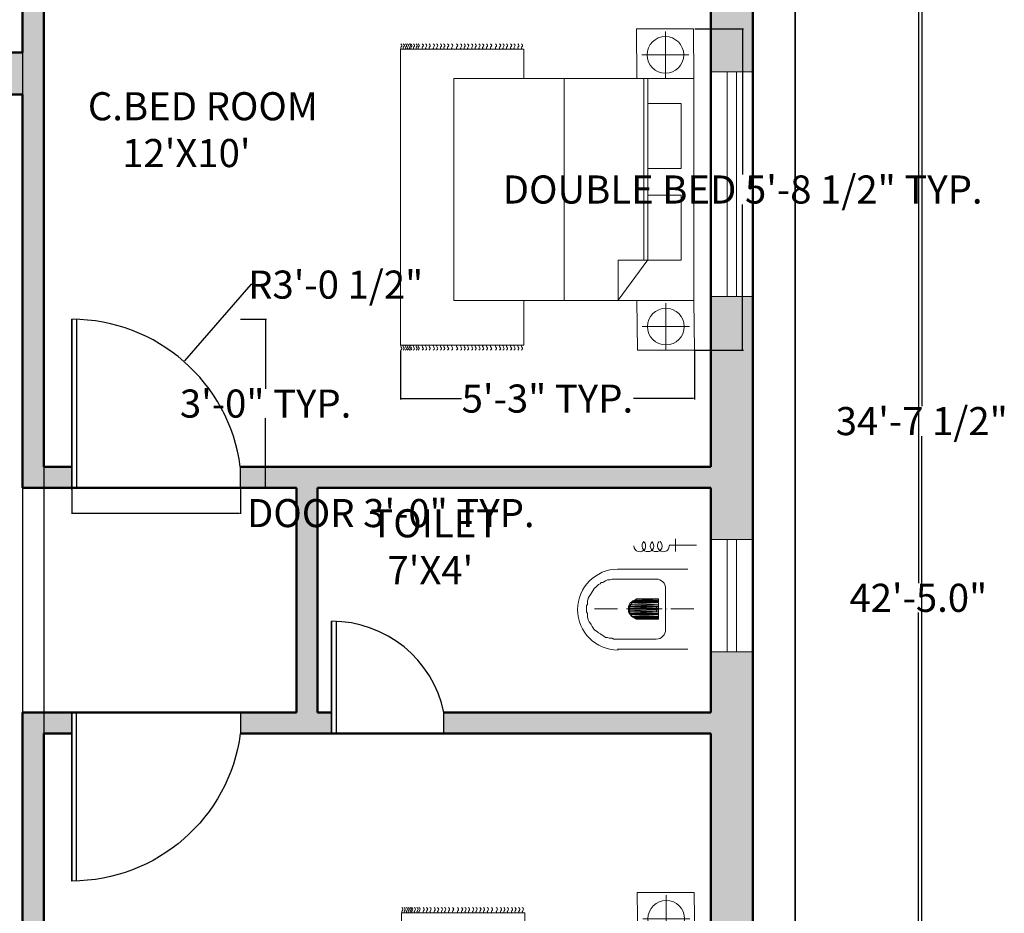
# Model space of a CAD drawing. Units: inches. Extents: x 3398 to 3816, y 15195 to 15771.
# Tile 8 of 10: x 3606 to 3816, y 15418 to 15609. Entities that reach past the tile are written whole.
import ezdxf

# ---------------------------------------------------------------- set-up
doc = ezdxf.new("R2010")
doc.units = ezdxf.units.IN
doc.header["$MEASUREMENT"] = 0
for name, color, linetype, lineweight in [('A-ANNO-DIMS', 2, 'Continuous', 18), ('A-AREA-IDEN', 7, 'Continuous', 25), ('A-DOOR', 3, 'Continuous', 25), ('A-FLOR-FIXT', 8, 'Continuous', 18), ('A-FURN', 8, 'Continuous', 18), ('A-GLAZ', 4, 'Continuous', 18), ('A-WALL', 7, 'Continuous', 50), ('A-WALL-PATT', 252, 'Continuous', 13), ('C-PROP', 7, 'Continuous', 35)]:
    doc.layers.add(name, color=color, linetype=linetype, lineweight=lineweight)
doc.styles.get("Standard").update_dxf_attribs({"font": 'arial.ttf'})
doc.dimstyles.get("Standard").update_dxf_attribs({"dimtxt": 6, "dimasz": 0.18, "dimexe": 0.18, "dimexo": 0.0625, "dimgap": 0.09, "dimtad": 0, "dimtih": 1, "dimtoh": 1, "dimdec": 1, "dimzin": 0, "dimdsep": 46, "dimlunit": 3, "dimtxsty": 'Standard', "dimcen": 0.09, "dimadec": 0, "dimazin": 0, "dimtfac": 1, "dimtdec": 1, "dimtofl": 0, "dimtmove": 0, "dimatfit": 3, "dimfxl": 1, "dimtolj": 1, "dimtzin": 0, "dimarcsym": 0})

# ---------------------------------------------------------------- blocks, each defined once
blk = doc.blocks.new('*D5')
at = {"layer": 'A-ANNO-DIMS', "color": 0, "lineweight": -2, "transparency": 16777216}
for p, q in [((3771.25, 15739.52), (3797.69, 15739.52)), ((3797.51, 15739.34), (3797.51, 15488.17)), ((3797.51, 15230.7), (3797.51, 15481.87)), ((3771.25, 15230.52), (3797.69, 15230.52))]:
    blk.add_line(p, q, dxfattribs=at)
at = {"layer": 'A-ANNO-DIMS', "color": 0, "transparency": 16777216}
for points in [[(3797.48, 15739.34), (3797.54, 15739.34), (3797.51, 15739.52)], [(3797.48, 15230.7), (3797.54, 15230.7), (3797.51, 15230.52)]]:
    blk.add_solid(points, dxfattribs=at)
at = {"layer": 'Defpoints', "color": 0, "transparency": 16777216}
for p in [(3771.19, 15739.52), (3771.19, 15230.52), (3797.51, 15230.52)]:
    blk.add_point(p, dxfattribs=at)
at = {"layer": 'A-ANNO-DIMS', "color": 0, "transparency": 16777216, "insert": (3797.51, 15485.02), "char_height": 6, "attachment_point": 5}
blk.add_mtext('\\A1;42\'-5.0"', dxfattribs=at)
blk = doc.blocks.new('BED-DOUBLE-WITH-NIGHTSTANDS')
for p, q in [((56.59, 58.08), (56.59, 68.14)), ((0, 64.36), (26.37, 64.36)), ((0, 1.12), (0, 64.36)), ((26.37, 64.36), (26.37, 58.06)), ((61.62, 63.11), (51.56, 63.11)), ((34.96, 10.66), (34.96, 58.08)), ((52, 19.27), (52, 58.08)), ((52.82, 19.32), (52.82, 58.08)), ((52.82, 19.32), (46.47, 10.71)), ((52.82, 19.27), (46.47, 19.27)), ((46.47, 19.27), (46.47, 10.71)), ((26.37, 10.66), (26.37, 1.12)), ((56.69, 0.03), (56.69, 10.09)), ((61.72, 5.06), (51.66, 5.06)), ((26.37, 1.12), (0, 1.12))]:
    blk.add_line(p, q)
for points in [[(50.39, 68.71), (50.5, 58.08), (62.68, 58.08), (62.58, 68.71)], [(62.68, 10.66), (11.37, 10.66), (11.37, 58.08), (62.68, 58.08)], [(59.98, 38.83), (52.82, 38.83), (52.82, 52.73), (59.98, 52.73)], [(59.98, 19.27), (52.82, 19.27), (52.82, 33.16), (59.98, 33.16)], [(50.5, 10.66), (50.6, 0.03), (62.78, 0.03), (62.68, 10.66)]]:
    blk.add_lwpolyline(points, close=True)
for centre in [(56.59, 63.11), (56.69, 5.06)]:
    blk.add_circle(centre, 3.92)
for points, knots in [([(0.07, 65.48), (0.19, 65.39), (0.43, 65.19), (0.19, 64.85), (0.02, 64.57), (0.13, 64.42), (0.18, 64.36)], [0, 0, 0, 0, 0.400747, 0.791423, 1.067667, 1.29709, 1.29709, 1.29709, 1.29709]), ([(0.57, 65.48), (0.7, 65.39), (0.94, 65.19), (0.7, 64.85), (0.52, 64.57), (0.63, 64.42), (0.68, 64.36)], [0, 0, 0, 0, 0.400747, 0.791423, 1.067667, 1.29709, 1.29709, 1.29709, 1.29709]), ([(1.06, 65.48), (1.18, 65.39), (1.42, 65.19), (1.18, 64.85), (1.01, 64.57), (1.11, 64.42), (1.16, 64.36)], [0, 0, 0, 0, 0.400747, 0.791423, 1.067667, 1.29709, 1.29709, 1.29709, 1.29709]), ([(1.46, 65.48), (1.58, 65.39), (1.82, 65.19), (1.58, 64.85), (1.41, 64.57), (1.51, 64.42), (1.56, 64.36)], [0, 0, 0, 0, 0.400747, 0.791423, 1.067667, 1.29709, 1.29709, 1.29709, 1.29709]), ([(1.88, 65.48), (2, 65.39), (2.24, 65.19), (2, 64.85), (1.82, 64.57), (1.93, 64.42), (1.98, 64.36)], [0, 0, 0, 0, 0.400747, 0.791423, 1.067667, 1.29709, 1.29709, 1.29709, 1.29709]), ([(2.18, 65.48), (2.31, 65.39), (2.55, 65.19), (2.31, 64.85), (2.13, 64.57), (2.24, 64.42), (2.29, 64.36)], [0, 0, 0, 0, 0.400747, 0.791423, 1.067667, 1.29709, 1.29709, 1.29709, 1.29709]), ([(2.76, 65.48), (2.88, 65.39), (3.12, 65.19), (2.88, 64.85), (2.71, 64.57), (2.81, 64.42), (2.86, 64.36)], [0, 0, 0, 0, 0.400747, 0.791423, 1.067667, 1.29709, 1.29709, 1.29709, 1.29709]), ([(3.33, 65.48), (3.45, 65.39), (3.7, 65.2), (3.44, 64.85), (3.27, 64.57), (3.38, 64.42), (3.43, 64.36)], [0, 0, 0, 0, 0.407265, 0.802015, 1.07826, 1.307683, 1.307683, 1.307683, 1.307683]), ([(3.75, 65.48), (3.88, 65.39), (4.12, 65.19), (3.88, 64.85), (3.7, 64.57), (3.81, 64.42), (3.86, 64.36)], [0, 0, 0, 0, 0.400747, 0.791423, 1.067667, 1.29709, 1.29709, 1.29709, 1.29709]), ([(4.64, 65.48), (4.76, 65.39), (5, 65.19), (4.76, 64.85), (4.59, 64.57), (4.69, 64.42), (4.74, 64.36)], [0, 0, 0, 0, 0.400747, 0.791423, 1.067667, 1.29709, 1.29709, 1.29709, 1.29709]), ([(5.36, 65.48), (5.49, 65.39), (5.73, 65.19), (5.49, 64.85), (5.31, 64.57), (5.42, 64.42), (5.47, 64.36)], [0, 0, 0, 0, 0.400747, 0.791423, 1.067667, 1.29709, 1.29709, 1.29709, 1.29709]), ([(6.12, 65.48), (6.24, 65.39), (6.48, 65.19), (6.24, 64.85), (6.07, 64.57), (6.17, 64.42), (6.22, 64.36)], [0, 0, 0, 0, 0.400747, 0.791423, 1.067667, 1.29709, 1.29709, 1.29709, 1.29709]), ([(7, 65.48), (7.12, 65.39), (7.36, 65.19), (7.12, 64.85), (6.95, 64.57), (7.05, 64.42), (7.1, 64.36)], [0, 0, 0, 0, 0.400747, 0.791423, 1.067667, 1.29709, 1.29709, 1.29709, 1.29709]), ([(7.73, 65.48), (7.85, 65.39), (8.09, 65.19), (7.85, 64.85), (7.68, 64.57), (7.78, 64.42), (7.83, 64.36)], [0, 0, 0, 0, 0.400747, 0.791423, 1.067667, 1.29709, 1.29709, 1.29709, 1.29709]), ([(8.54, 65.48), (8.66, 65.39), (8.9, 65.19), (8.66, 64.85), (8.49, 64.57), (8.6, 64.42), (8.65, 64.36)], [0, 0, 0, 0, 0.400747, 0.791423, 1.067667, 1.29709, 1.29709, 1.29709, 1.29709]), ([(9.23, 65.48), (9.35, 65.39), (9.59, 65.19), (9.35, 64.85), (9.18, 64.57), (9.29, 64.42), (9.34, 64.36)], [0, 0, 0, 0, 0.400747, 0.791423, 1.067667, 1.29709, 1.29709, 1.29709, 1.29709]), ([(10.05, 65.48), (10.17, 65.39), (10.41, 65.19), (10.17, 64.85), (10, 64.57), (10.1, 64.42), (10.15, 64.36)], [0, 0, 0, 0, 0.400747, 0.791423, 1.067667, 1.29709, 1.29709, 1.29709, 1.29709]), ([(10.93, 65.48), (11.05, 65.39), (11.29, 65.19), (11.05, 64.85), (10.88, 64.57), (10.99, 64.42), (11.03, 64.36)], [0, 0, 0, 0, 0.400747, 0.791423, 1.067667, 1.29709, 1.29709, 1.29709, 1.29709]), ([(11.97, 65.48), (12.09, 65.39), (12.33, 65.19), (12.09, 64.85), (11.92, 64.57), (12.02, 64.42), (12.07, 64.36)], [0, 0, 0, 0, 0.400747, 0.791423, 1.067667, 1.29709, 1.29709, 1.29709, 1.29709]), ([(12.85, 65.48), (12.97, 65.39), (13.21, 65.19), (12.97, 64.85), (12.8, 64.57), (12.9, 64.42), (12.95, 64.36)], [0, 0, 0, 0, 0.400747, 0.791423, 1.067667, 1.29709, 1.29709, 1.29709, 1.29709]), ([(13.58, 65.48), (13.7, 65.39), (13.94, 65.19), (13.7, 64.85), (13.53, 64.57), (13.63, 64.42), (13.68, 64.36)], [0, 0, 0, 0, 0.400747, 0.791423, 1.067667, 1.29709, 1.29709, 1.29709, 1.29709]), ([(14.33, 65.48), (14.45, 65.39), (14.69, 65.19), (14.45, 64.85), (14.28, 64.57), (14.38, 64.42), (14.43, 64.36)], [0, 0, 0, 0, 0.400747, 0.791423, 1.067667, 1.29709, 1.29709, 1.29709, 1.29709]), ([(15.21, 65.48), (15.33, 65.39), (15.57, 65.19), (15.33, 64.85), (15.16, 64.57), (15.27, 64.42), (15.32, 64.36)], [0, 0, 0, 0, 0.400747, 0.791423, 1.067667, 1.29709, 1.29709, 1.29709, 1.29709]), ([(15.94, 65.48), (16.06, 65.39), (16.3, 65.19), (16.06, 64.85), (15.89, 64.57), (16, 64.42), (16.04, 64.36)], [0, 0, 0, 0, 0.400747, 0.791423, 1.067667, 1.29709, 1.29709, 1.29709, 1.29709]), ([(16.76, 65.48), (16.88, 65.39), (17.12, 65.19), (16.88, 64.85), (16.7, 64.57), (16.81, 64.42), (16.86, 64.36)], [0, 0, 0, 0, 0.400747, 0.791423, 1.067667, 1.29709, 1.29709, 1.29709, 1.29709]), ([(17.53, 65.48), (17.65, 65.39), (17.89, 65.19), (17.65, 64.85), (17.48, 64.57), (17.59, 64.42), (17.64, 64.36)], [0, 0, 0, 0, 0.400747, 0.791423, 1.067667, 1.29709, 1.29709, 1.29709, 1.29709]), ([(18.35, 65.48), (18.47, 65.39), (18.71, 65.19), (18.47, 64.85), (18.3, 64.57), (18.4, 64.42), (18.45, 64.36)], [0, 0, 0, 0, 0.400747, 0.791423, 1.067667, 1.29709, 1.29709, 1.29709, 1.29709]), ([(19.23, 65.48), (19.35, 65.39), (19.59, 65.19), (19.35, 64.85), (19.18, 64.57), (19.29, 64.42), (19.33, 64.36)], [0, 0, 0, 0, 0.400747, 0.791423, 1.067667, 1.29709, 1.29709, 1.29709, 1.29709]), ([(20.27, 65.48), (20.39, 65.39), (20.63, 65.19), (20.39, 64.85), (20.22, 64.57), (20.32, 64.42), (20.37, 64.36)], [0, 0, 0, 0, 0.400747, 0.791423, 1.067667, 1.29709, 1.29709, 1.29709, 1.29709]), ([(21.15, 65.48), (21.27, 65.39), (21.51, 65.19), (21.27, 64.85), (21.1, 64.57), (21.21, 64.42), (21.25, 64.36)], [0, 0, 0, 0, 0.400747, 0.791423, 1.067667, 1.29709, 1.29709, 1.29709, 1.29709]), ([(21.88, 65.48), (22, 65.39), (22.24, 65.19), (22, 64.85), (21.83, 64.57), (21.93, 64.42), (21.98, 64.36)], [0, 0, 0, 0, 0.400747, 0.791423, 1.067667, 1.29709, 1.29709, 1.29709, 1.29709]), ([(22.63, 65.48), (22.75, 65.39), (22.99, 65.19), (22.75, 64.85), (22.58, 64.57), (22.69, 64.42), (22.73, 64.36)], [0, 0, 0, 0, 0.400747, 0.791423, 1.067667, 1.29709, 1.29709, 1.29709, 1.29709]), ([(23.51, 65.48), (23.63, 65.39), (23.87, 65.19), (23.63, 64.85), (23.46, 64.57), (23.57, 64.42), (23.62, 64.36)], [0, 0, 0, 0, 0.400747, 0.791423, 1.067667, 1.29709, 1.29709, 1.29709, 1.29709]), ([(24.24, 65.48), (24.36, 65.39), (24.6, 65.19), (24.36, 64.85), (24.19, 64.57), (24.3, 64.42), (24.34, 64.36)], [0, 0, 0, 0, 0.400747, 0.791423, 1.067667, 1.29709, 1.29709, 1.29709, 1.29709]), ([(25.06, 65.48), (25.18, 65.39), (25.42, 65.19), (25.18, 64.85), (25.01, 64.57), (25.11, 64.42), (25.16, 64.36)], [0, 0, 0, 0, 0.400747, 0.791423, 1.067667, 1.29709, 1.29709, 1.29709, 1.29709]), ([(25.84, 65.48), (25.96, 65.39), (26.2, 65.19), (25.96, 64.85), (25.78, 64.57), (25.89, 64.42), (25.94, 64.36)], [0, 0, 0, 0, 0.400747, 0.791423, 1.067667, 1.29709, 1.29709, 1.29709, 1.29709]), ([(0.07, 0), (0.19, 0.1), (0.43, 0.29), (0.19, 0.63), (0.02, 0.91), (0.13, 1.06), (0.18, 1.13)], [0, 0, 0, 0, 0.400747, 0.791423, 1.067667, 1.29709, 1.29709, 1.29709, 1.29709]), ([(0.55, 0), (0.67, 0.1), (0.91, 0.29), (0.67, 0.63), (0.49, 0.91), (0.6, 1.06), (0.65, 1.13)], [0, 0, 0, 0, 0.400747, 0.791423, 1.067667, 1.29709, 1.29709, 1.29709, 1.29709]), ([(1.03, 0), (1.15, 0.1), (1.39, 0.29), (1.15, 0.63), (0.98, 0.91), (1.09, 1.06), (1.13, 1.13)], [0, 0, 0, 0, 0.400747, 0.791423, 1.067667, 1.29709, 1.29709, 1.29709, 1.29709]), ([(1.43, 0), (1.55, 0.1), (1.79, 0.29), (1.55, 0.63), (1.38, 0.91), (1.48, 1.06), (1.53, 1.13)], [0, 0, 0, 0, 0.400747, 0.791423, 1.067667, 1.29709, 1.29709, 1.29709, 1.29709]), ([(1.85, 0), (1.97, 0.1), (2.21, 0.29), (1.97, 0.63), (1.8, 0.91), (1.9, 1.05), (1.94, 1.12)], [0, 0, 0, 0, 0.400747, 0.791423, 1.067667, 1.283686, 1.283686, 1.283686, 1.283686]), ([(2.16, 0), (2.28, 0.1), (2.52, 0.29), (2.28, 0.63), (2.11, 0.91), (2.21, 1.05), (2.25, 1.12)], [0, 0, 0, 0, 0.400747, 0.791423, 1.067667, 1.283686, 1.283686, 1.283686, 1.283686]), ([(2.73, 0), (2.85, 0.1), (3.09, 0.29), (2.85, 0.63), (2.68, 0.91), (2.78, 1.05), (2.82, 1.12)], [0, 0, 0, 0, 0.400747, 0.791423, 1.067667, 1.283686, 1.283686, 1.283686, 1.283686]), ([(3.33, 0), (3.45, 0.1), (3.69, 0.29), (3.45, 0.63), (3.27, 0.91), (3.38, 1.05), (3.42, 1.12)], [0, 0, 0, 0, 0.402903, 0.794912, 1.071156, 1.287177, 1.287177, 1.287177, 1.287177]), ([(3.75, 0), (3.88, 0.1), (4.11, 0.29), (3.88, 0.63), (3.7, 0.91), (3.81, 1.05), (3.85, 1.12)], [0, 0, 0, 0, 0.400747, 0.791423, 1.067667, 1.283686, 1.283686, 1.283686, 1.283686]), ([(4.64, 0), (4.76, 0.1), (5, 0.29), (4.76, 0.63), (4.59, 0.91), (4.69, 1.05), (4.73, 1.12)], [0, 0, 0, 0, 0.400747, 0.791423, 1.067667, 1.283686, 1.283686, 1.283686, 1.283686]), ([(5.36, 0), (5.49, 0.1), (5.73, 0.29), (5.49, 0.63), (5.31, 0.91), (5.42, 1.06), (5.47, 1.13)], [0, 0, 0, 0, 0.400747, 0.791423, 1.067667, 1.29709, 1.29709, 1.29709, 1.29709]), ([(6.12, 0), (6.24, 0.1), (6.48, 0.29), (6.24, 0.63), (6.07, 0.91), (6.17, 1.06), (6.22, 1.13)], [0, 0, 0, 0, 0.400747, 0.791423, 1.067667, 1.29709, 1.29709, 1.29709, 1.29709]), ([(7, 0), (7.12, 0.1), (7.36, 0.29), (7.12, 0.63), (6.95, 0.91), (7.05, 1.06), (7.1, 1.13)], [0, 0, 0, 0, 0.400747, 0.791423, 1.067667, 1.29709, 1.29709, 1.29709, 1.29709]), ([(7.73, 0), (7.85, 0.1), (8.09, 0.29), (7.85, 0.63), (7.68, 0.91), (7.78, 1.06), (7.83, 1.13)], [0, 0, 0, 0, 0.400747, 0.791423, 1.067667, 1.29709, 1.29709, 1.29709, 1.29709]), ([(8.54, 0), (8.66, 0.1), (8.9, 0.29), (8.66, 0.63), (8.49, 0.91), (8.6, 1.06), (8.65, 1.13)], [0, 0, 0, 0, 0.400747, 0.791423, 1.067667, 1.29709, 1.29709, 1.29709, 1.29709]), ([(9.23, 0), (9.35, 0.1), (9.59, 0.29), (9.35, 0.63), (9.18, 0.91), (9.29, 1.06), (9.34, 1.13)], [0, 0, 0, 0, 0.400747, 0.791423, 1.067667, 1.29709, 1.29709, 1.29709, 1.29709]), ([(10.05, 0), (10.17, 0.1), (10.41, 0.29), (10.17, 0.63), (10, 0.91), (10.1, 1.06), (10.15, 1.13)], [0, 0, 0, 0, 0.400747, 0.791423, 1.067667, 1.29709, 1.29709, 1.29709, 1.29709]), ([(10.93, 0), (11.05, 0.1), (11.29, 0.29), (11.05, 0.63), (10.88, 0.91), (10.99, 1.06), (11.03, 1.13)], [0, 0, 0, 0, 0.400747, 0.791423, 1.067667, 1.29709, 1.29709, 1.29709, 1.29709]), ([(11.97, 0), (12.09, 0.1), (12.33, 0.29), (12.09, 0.63), (11.92, 0.91), (12.02, 1.06), (12.07, 1.13)], [0, 0, 0, 0, 0.400747, 0.791423, 1.067667, 1.29709, 1.29709, 1.29709, 1.29709]), ([(12.85, 0), (12.97, 0.1), (13.21, 0.29), (12.97, 0.63), (12.8, 0.91), (12.9, 1.06), (12.95, 1.13)], [0, 0, 0, 0, 0.400747, 0.791423, 1.067667, 1.29709, 1.29709, 1.29709, 1.29709]), ([(13.58, 0), (13.7, 0.1), (13.94, 0.29), (13.7, 0.63), (13.53, 0.91), (13.63, 1.06), (13.68, 1.13)], [0, 0, 0, 0, 0.400747, 0.791423, 1.067667, 1.29709, 1.29709, 1.29709, 1.29709]), ([(14.33, 0), (14.45, 0.1), (14.69, 0.29), (14.45, 0.63), (14.28, 0.91), (14.38, 1.06), (14.43, 1.13)], [0, 0, 0, 0, 0.400747, 0.791423, 1.067667, 1.29709, 1.29709, 1.29709, 1.29709]), ([(15.21, 0), (15.33, 0.1), (15.57, 0.29), (15.33, 0.63), (15.16, 0.91), (15.27, 1.06), (15.32, 1.13)], [0, 0, 0, 0, 0.400747, 0.791423, 1.067667, 1.29709, 1.29709, 1.29709, 1.29709]), ([(15.94, 0), (16.06, 0.1), (16.3, 0.29), (16.06, 0.63), (15.89, 0.91), (16, 1.06), (16.04, 1.13)], [0, 0, 0, 0, 0.400747, 0.791423, 1.067667, 1.29709, 1.29709, 1.29709, 1.29709]), ([(16.76, 0), (16.88, 0.1), (17.12, 0.29), (16.88, 0.63), (16.7, 0.91), (16.81, 1.06), (16.86, 1.13)], [0, 0, 0, 0, 0.400747, 0.791423, 1.067667, 1.29709, 1.29709, 1.29709, 1.29709]), ([(17.53, 0), (17.65, 0.1), (17.89, 0.29), (17.65, 0.63), (17.48, 0.91), (17.59, 1.06), (17.64, 1.13)], [0, 0, 0, 0, 0.400747, 0.791423, 1.067667, 1.29709, 1.29709, 1.29709, 1.29709]), ([(18.35, 0), (18.47, 0.1), (18.71, 0.29), (18.47, 0.63), (18.3, 0.91), (18.4, 1.06), (18.45, 1.13)], [0, 0, 0, 0, 0.400747, 0.791423, 1.067667, 1.29709, 1.29709, 1.29709, 1.29709]), ([(19.23, 0), (19.35, 0.1), (19.59, 0.29), (19.35, 0.63), (19.18, 0.91), (19.29, 1.06), (19.33, 1.13)], [0, 0, 0, 0, 0.400747, 0.791423, 1.067667, 1.29709, 1.29709, 1.29709, 1.29709]), ([(20.27, 0), (20.39, 0.1), (20.63, 0.29), (20.39, 0.63), (20.22, 0.91), (20.32, 1.06), (20.37, 1.13)], [0, 0, 0, 0, 0.400747, 0.791423, 1.067667, 1.29709, 1.29709, 1.29709, 1.29709]), ([(21.15, 0), (21.27, 0.1), (21.51, 0.29), (21.27, 0.63), (21.1, 0.91), (21.21, 1.06), (21.25, 1.13)], [0, 0, 0, 0, 0.400747, 0.791423, 1.067667, 1.29709, 1.29709, 1.29709, 1.29709]), ([(21.88, 0), (22, 0.1), (22.24, 0.29), (22, 0.63), (21.83, 0.91), (21.93, 1.06), (21.98, 1.13)], [0, 0, 0, 0, 0.400747, 0.791423, 1.067667, 1.29709, 1.29709, 1.29709, 1.29709]), ([(22.63, 0), (22.75, 0.1), (22.99, 0.29), (22.75, 0.63), (22.58, 0.91), (22.69, 1.06), (22.73, 1.13)], [0, 0, 0, 0, 0.400747, 0.791423, 1.067667, 1.29709, 1.29709, 1.29709, 1.29709]), ([(23.51, 0), (23.63, 0.1), (23.87, 0.29), (23.63, 0.63), (23.46, 0.91), (23.57, 1.06), (23.62, 1.13)], [0, 0, 0, 0, 0.400747, 0.791423, 1.067667, 1.29709, 1.29709, 1.29709, 1.29709]), ([(24.24, 0), (24.36, 0.1), (24.6, 0.29), (24.36, 0.63), (24.19, 0.91), (24.3, 1.06), (24.34, 1.13)], [0, 0, 0, 0, 0.400747, 0.791423, 1.067667, 1.29709, 1.29709, 1.29709, 1.29709]), ([(25.06, 0), (25.18, 0.1), (25.42, 0.29), (25.18, 0.63), (25.01, 0.91), (25.11, 1.06), (25.16, 1.13)], [0, 0, 0, 0, 0.400747, 0.791423, 1.067667, 1.29709, 1.29709, 1.29709, 1.29709]), ([(25.84, 0), (25.96, 0.1), (26.2, 0.29), (25.96, 0.63), (25.78, 0.91), (25.89, 1.06), (25.94, 1.13)], [0, 0, 0, 0, 0.400747, 0.791423, 1.067667, 1.29709, 1.29709, 1.29709, 1.29709])]:
    blk.add_open_spline(points, degree=3, knots=knots)
blk = doc.blocks.new('WC-PLAN')
h = blk.add_hatch(color=256)
h.paths.add_polyline_path([(12.84, 17.3), (12.84, 12.59), (13.07, 17.3)])
h.paths.add_polyline_path([(12.84, 12.59), (13.07, 17.3), (13.07, 12.21)])
h = blk.add_hatch(color=256)
h.paths.add_polyline_path([(13.07, 17.3), (13.07, 12.21), (13.22, 17.3)])
h.paths.add_polyline_path([(13.07, 12.21), (13.22, 17.3), (13.22, 11.83)])
h = blk.add_hatch(color=256)
h.paths.add_polyline_path([(13.22, 17.3), (13.22, 11.83), (13.45, 17.3)])
h.paths.add_polyline_path([(13.22, 11.83), (13.45, 17.3), (13.45, 11.61)])
h = blk.add_hatch(color=256)
h.paths.add_polyline_path([(13.45, 17.3), (13.45, 11.61), (13.6, 17.3)])
h.paths.add_polyline_path([(13.45, 11.61), (13.6, 17.3), (13.6, 11.23)])
h = blk.add_hatch(color=256)
h.paths.add_polyline_path([(13.6, 17.3), (13.6, 11.23), (14.06, 17.3)])
h.paths.add_polyline_path([(13.6, 11.23), (14.06, 17.3), (14.06, 11.08)])
h = blk.add_hatch(color=256)
h.paths.add_polyline_path([(14.06, 17.3), (14.06, 11.08), (14.44, 17.3)])
h.paths.add_polyline_path([(14.06, 11.08), (14.44, 17.3), (14.44, 10.85)])
h = blk.add_hatch(color=256)
h.paths.add_polyline_path([(14.44, 17.3), (14.44, 10.85), (14.82, 17.3)])
h.paths.add_polyline_path([(14.44, 10.85), (14.82, 17.3), (14.82, 10.85)])
h = blk.add_hatch(color=256)
h.paths.add_polyline_path([(14.82, 17.3), (14.82, 10.85), (15.19, 17.3)])
h.paths.add_polyline_path([(14.82, 10.85), (15.19, 17.3), (15.2, 10.85)])
h = blk.add_hatch(color=256)
h.paths.add_polyline_path([(15.19, 17.3), (15.2, 10.85), (15.57, 17.3)])
h.paths.add_polyline_path([(15.2, 10.85), (15.57, 17.3), (15.58, 10.85)])
h = blk.add_hatch(color=256)
h.paths.add_polyline_path([(15.57, 17.3), (15.58, 10.85), (15.95, 17.3)])
h.paths.add_polyline_path([(15.58, 10.85), (15.95, 17.3), (15.96, 11.08)])
h = blk.add_hatch(color=256)
h.paths.add_polyline_path([(15.95, 17.3), (15.96, 11.08), (16.18, 17.3)])
h.paths.add_polyline_path([(15.96, 11.08), (16.18, 17.3), (16.18, 11.23)])
h = blk.add_hatch(color=256)
h.paths.add_polyline_path([(16.18, 17.3), (16.18, 11.23), (16.56, 17.3)])
h.paths.add_polyline_path([(16.18, 11.23), (16.56, 17.3), (16.56, 11.61)])
h = blk.add_hatch(color=256)
h.paths.add_polyline_path([(16.56, 17.3), (16.56, 11.61), (16.71, 17.3)])
h.paths.add_polyline_path([(16.56, 11.61), (16.71, 17.3), (16.71, 11.83)])
h = blk.add_hatch(color=256)
h.paths.add_polyline_path([(16.71, 17.3), (16.71, 11.83), (16.94, 17.3)])
h.paths.add_polyline_path([(16.71, 11.83), (16.94, 17.3), (16.94, 12.21)])
h = blk.add_hatch(color=256)
h.paths.add_polyline_path([(16.94, 17.3), (16.94, 12.21), (17.17, 17.3)])
h.paths.add_polyline_path([(16.94, 12.21), (17.17, 17.3), (17.17, 12.59)])
h.paths.add_polyline_path([(17.17, 17.3), (17.17, 12.59), (17.17, 12.97)])
for points in [[(1.36, 25.41), (1.37, 19.57), (1.37, 19.57)], [(6.47, 23.51), (6.47, 8.49), (6.47, 8.49)], [(14.97, 24.81), (14.97, 19.95), (14.97, 19.95)], [(23.54, 23.52), (23.54, 8.5), (23.54, 8.5)], [(2.73, 20.93), (0, 20.93), (0, 20.93)], [(14.97, 19.04), (15.04, 19.04), (15.04, 19.04)], [(19.29, 18.81), (10.57, 18.81), (10.57, 18.81)], [(17.17, 17.3), (12.84, 17.3), (12.84, 17.3)], [(12.84, 17.3), (12.84, 12.97), (12.84, 12.97)], [(14.59, 16.84), (14.59, 16.92), (14.59, 16.92)], [(14.97, 16.84), (14.82, 16.84), (14.59, 16.84)], [(14.97, 18.05), (14.97, 10.47), (14.97, 10.47)], [(14.97, 16.84), (15.04, 16.92), (15.04, 16.92)], [(15.42, 16.84), (15.2, 16.84), (14.97, 16.84)], [(15.42, 16.84), (15.42, 16.92), (15.42, 16.92)], [(17.17, 17.3), (17.17, 12.97), (17.17, 12.97)], [(8.6, 16.69), (8.6, 9.48), (8.6, 9.48)], [(21.42, 16.69), (21.42, 9.48), (21.42, 9.48)], [(21.42, 9.48), (21.42, 8.73), (21.42, 8.12), (21.42, 7.74), (21.19, 7.36), (21.19, 6.98), (21.19, 6.75), (21.04, 6.37), (21.04, 5.99), (20.81, 5.62), (20.66, 5.39), (20.43, 5.01), (20.28, 4.86), (20.05, 4.48), (19.83, 4.25), (19.67, 3.87), (19.45, 3.64), (19.29, 3.49), (18.92, 3.26), (18.69, 3.11), (18.31, 2.88), (18.08, 2.73), (17.7, 2.5), (17.32, 2.28), (17.17, 2.28), (16.72, 2.12), (16.34, 2.12), (15.96, 2.12), (15.58, 1.9), (14.97, 1.9), (14.21, 1.9), (14.06, 2.12), (13.61, 2.12), (13.23, 2.12), (12.85, 2.28), (12.7, 2.28), (12.32, 2.5), (11.86, 2.73), (11.71, 2.88), (11.33, 3.11), (11.1, 3.26), (10.72, 3.49), (10.57, 3.64), (10.34, 3.87), (9.96, 4.25), (9.74, 4.47), (9.58, 4.85), (9.36, 5.01), (9.36, 5.38), (9.21, 5.61), (8.98, 5.99), (8.75, 6.37), (8.75, 6.75), (8.75, 6.98), (8.6, 7.36), (8.6, 7.74), (8.6, 8.12), (8.6, 8.72), (8.6, 9.48)], [(14.97, 8.5), (14.97, 3.64), (14.97, 3.64)]]:
    blk.add_lwpolyline(points)
for points in [[(12.84, 17.3), (12.84, 12.97)], [(12.84, 12.97), (12.84, 17.3), (12.84, 12.59)], [(12.84, 17.3), (12.84, 12.59), (13.07, 17.3)], [(12.84, 12.59), (13.07, 17.3), (13.07, 12.21)], [(13.07, 17.3), (13.07, 12.21), (13.22, 17.3)], [(13.07, 12.21), (13.22, 17.3), (13.22, 11.83)], [(13.22, 17.3), (13.22, 11.83), (13.45, 17.3)], [(13.22, 11.83), (13.45, 17.3), (13.45, 11.61)], [(13.45, 17.3), (13.45, 11.61), (13.6, 17.3)], [(13.45, 11.61), (13.6, 17.3), (13.6, 11.23)], [(13.6, 17.3), (13.6, 11.23), (14.06, 17.3)], [(13.6, 11.23), (14.06, 17.3), (14.06, 11.08)], [(14.06, 17.3), (14.06, 11.08), (14.44, 17.3)], [(14.06, 11.08), (14.44, 17.3), (14.44, 10.85)], [(14.44, 17.3), (14.44, 10.85), (14.82, 17.3)], [(14.44, 10.85), (14.82, 17.3), (14.82, 10.85)], [(14.82, 17.3), (14.82, 10.85), (15.19, 17.3)], [(14.82, 10.85), (15.19, 17.3), (15.2, 10.85)], [(15.19, 17.3), (15.2, 10.85), (15.57, 17.3)], [(15.2, 10.85), (15.57, 17.3), (15.58, 10.85)], [(15.57, 17.3), (15.58, 10.85), (15.95, 17.3)], [(15.58, 10.85), (15.95, 17.3), (15.96, 11.08)], [(15.95, 17.3), (15.96, 11.08), (16.18, 17.3)], [(15.96, 11.08), (16.18, 17.3), (16.18, 11.23)], [(16.18, 17.3), (16.18, 11.23), (16.56, 17.3)], [(16.18, 11.23), (16.56, 17.3), (16.56, 11.61)], [(16.56, 17.3), (16.56, 11.61), (16.71, 17.3)], [(16.56, 11.61), (16.71, 17.3), (16.71, 11.83)], [(16.71, 17.3), (16.71, 11.83), (16.94, 17.3)], [(16.71, 11.83), (16.94, 17.3), (16.94, 12.21)], [(16.94, 17.3), (16.94, 12.21), (17.17, 17.3)], [(16.94, 12.21), (17.17, 17.3), (17.17, 12.59)], [(17.17, 17.3), (17.17, 12.59), (17.17, 12.97)], [(17.17, 12.59), (17.17, 17.3), (17.17, 17.3)]]:
    blk.add_lwpolyline(points, close=True)
for points, knots in [([(0.53, 17.44), (0.91, 17.06), (1.59, 16.91), (2.05, 17.22), (2.05, 17.22), (2.58, 17.52), (2.88, 18.05), (2.73, 18.66), (2.73, 18.66), (2.58, 19.19), (2.05, 19.57), (1.52, 19.57)], [0, 0, 0, 0, 0.083333, 0.083333, 0.083333, 0.083334, 0.166667, 0.166667, 0.166667, 0.166668, 1, 1, 1, 1]), ([(0.61, 15.93), (0.91, 15.55), (1.52, 15.4), (1.97, 15.62), (1.97, 15.62), (2.43, 15.78), (2.73, 16.31), (2.73, 16.76), (2.73, 16.76), (2.73, 17.29), (2.43, 17.75), (1.97, 17.97), (1.97, 17.97), (1.44, 18.13), (0.91, 17.97), (0.53, 17.6)], [0, 0, 0, 0, 0.0625, 0.0625, 0.0625, 0.062501, 0.125, 0.125, 0.125, 0.125001, 0.1875, 0.1875, 0.1875, 0.187501, 1, 1, 1, 1]), ([(0.53, 14.18), (0.91, 13.8), (1.44, 13.65), (1.97, 13.88), (1.97, 13.88), (2.43, 14.03), (2.73, 14.49), (2.73, 15.02), (2.73, 15.02), (2.73, 15.55), (2.43, 16), (1.97, 16.23), (1.97, 16.23), (1.44, 16.38), (0.91, 16.23), (0.53, 15.85)], [0, 0, 0, 0, 0.0625, 0.0625, 0.0625, 0.062501, 0.125, 0.125, 0.125, 0.125001, 0.1875, 0.1875, 0.1875, 0.187501, 1, 1, 1, 1]), ([(1.52, 11.98), (2.05, 11.98), (2.58, 12.44), (2.73, 12.97), (2.73, 12.97), (2.88, 13.5), (2.58, 14.11), (2.13, 14.41), (2.13, 14.41), (1.59, 14.64), (0.99, 14.56), (0.61, 14.18)], [0, 0, 0, 0, 0.083333, 0.083333, 0.083333, 0.083334, 0.166667, 0.166667, 0.166667, 0.166668, 1, 1, 1, 1]), ([(13.07, 13.12), (13.07, 11.99), (13.98, 11.08), (15.12, 11.08), (15.12, 11.08), (16.26, 11.08), (17.17, 11.99), (17.17, 13.12)], [0, 0, 0, 0, 0.125, 0.125, 0.125, 0.125001, 1, 1, 1, 1]), ([(6.47, 8.65), (6.47, 3.87), (10.34, 0), (15.12, 0), (15.12, 0), (19.9, 0), (23.77, 3.87), (23.77, 8.65)], [0, 0, 0, 0, 0.125, 0.125, 0.125, 0.125001, 1, 1, 1, 1])]:
    blk.add_open_spline(points, degree=3, knots=knots)
for points in [[(10.64, 18.81), (9.51, 18.81), (8.6, 17.9), (8.6, 16.76)], [(21.42, 16.77), (21.42, 17.9), (20.5, 18.81), (19.37, 18.81)]]:
    blk.add_open_spline(points, degree=3)
blk = doc.blocks.new('DOOR-SWING-36IN')
for p, q in [((0, 0), (0, 36)), ((1, 36), (1, 0)), ((0, 0), (36, 0))]:
    blk.add_line(p, q)
blk.add_arc((0, -0.32), 36.32, 7.6281, 90)
blk = doc.blocks.new('DOOR-SWING-24IN')
for p, q in [((0, 0), (0, 24)), ((1, 24), (1, 0)), ((0, 0), (24, 0))]:
    blk.add_line(p, q)
blk.add_arc((0, -0.52), 24.52, 11.8123, 90)
blk = doc.blocks.new('WINDOW-SASH-48IN')
for p, q in [((48, 9), (0, 9)), ((48, 5.5), (0, 5.5)), ((0, 3.5), (48, 3.5)), ((0, 0), (48, 0))]:
    blk.add_line(p, q)
blk = doc.blocks.new('*D22')
at = {"layer": 'A-ANNO-DIMS', "color": 0, "lineweight": -2, "transparency": 16777216}
for p, q in [((3749.74, 15606.61), (3760.16, 15606.61)), ((3759.98, 15606.43), (3759.98, 15575.44)), ((3759.98, 15538.08), (3759.98, 15569.06)), ((3749.74, 15537.9), (3760.16, 15537.9))]:
    blk.add_line(p, q, dxfattribs=at)
at = {"layer": 'A-ANNO-DIMS', "color": 0, "transparency": 16777216}
for points in [[(3759.95, 15606.43), (3760.01, 15606.43), (3759.98, 15606.61)], [(3759.95, 15538.08), (3760.01, 15538.08), (3759.98, 15537.9)]]:
    blk.add_solid(points, dxfattribs=at)
at = {"layer": 'Defpoints', "color": 0, "transparency": 16777216}
for p in [(3749.67, 15606.61), (3759.98, 15606.61), (3749.67, 15537.9)]:
    blk.add_point(p, dxfattribs=at)
at = {"layer": 'A-ANNO-DIMS', "color": 0, "transparency": 16777216, "insert": (3759.98, 15572.25), "char_height": 6, "attachment_point": 5}
blk.add_mtext('\\A1;DOUBLE BED 5\'-8 1/2" TYP.', dxfattribs=at)
blk = doc.blocks.new('*D23')
at = {"layer": 'A-ANNO-DIMS', "color": 0, "lineweight": -2, "transparency": 16777216}
for p, q in [((3686.89, 15537.83), (3686.89, 15527.41)), ((3749.67, 15537.83), (3749.67, 15527.41)), ((3687.07, 15527.59), (3699.91, 15527.59)), ((3749.49, 15527.59), (3736.66, 15527.59))]:
    blk.add_line(p, q, dxfattribs=at)
at = {"layer": 'A-ANNO-DIMS', "color": 0, "transparency": 16777216}
for points in [[(3687.07, 15527.62), (3687.07, 15527.56), (3686.89, 15527.59)], [(3749.49, 15527.62), (3749.49, 15527.56), (3749.67, 15527.59)]]:
    blk.add_solid(points, dxfattribs=at)
at = {"layer": 'Defpoints', "color": 0, "transparency": 16777216}
for p in [(3686.89, 15537.9), (3749.67, 15537.9), (3749.67, 15527.59)]:
    blk.add_point(p, dxfattribs=at)
at = {"layer": 'A-ANNO-DIMS', "color": 0, "transparency": 16777216, "insert": (3718.28, 15527.59), "char_height": 6, "attachment_point": 5}
blk.add_mtext('\\A1;5\'-3" TYP.', dxfattribs=at)
blk = doc.blocks.new('*D26')
at = {"layer": 'A-ANNO-DIMS', "color": 0, "lineweight": -2, "transparency": 16777216}
for p, q in [((3616.69, 15508.46), (3616.69, 15502.94)), ((3652.69, 15508.46), (3652.69, 15502.94)), ((3616.87, 15503.12), (3652.51, 15503.12)), ((3652.69, 15503.12), (3652.87, 15503.12))]:
    blk.add_line(p, q, dxfattribs=at)
at = {"layer": 'A-ANNO-DIMS', "color": 0, "transparency": 16777216}
for points in [[(3616.87, 15503.15), (3616.87, 15503.09), (3616.69, 15503.12)], [(3652.51, 15503.15), (3652.51, 15503.09), (3652.69, 15503.12)]]:
    blk.add_solid(points, dxfattribs=at)
at = {"layer": 'Defpoints', "color": 0, "transparency": 16777216}
for p in [(3616.69, 15508.52), (3652.69, 15508.52), (3652.69, 15503.12)]:
    blk.add_point(p, dxfattribs=at)
at = {"layer": 'A-ANNO-DIMS', "color": 0, "transparency": 16777216, "insert": (3684.83, 15503.12), "char_height": 6, "attachment_point": 5}
blk.add_mtext('\\A1;DOOR 3\'-0" TYP.', dxfattribs=at)
blk = doc.blocks.new('*D27')
at = {"layer": 'A-ANNO-DIMS', "color": 0, "lineweight": -2, "transparency": 16777216}
for p, q in [((3652.75, 15544.52), (3658.27, 15544.52)), ((3658.09, 15544.34), (3658.09, 15529.68)), ((3658.09, 15508.7), (3658.09, 15523.37)), ((3652.75, 15508.52), (3658.27, 15508.52))]:
    blk.add_line(p, q, dxfattribs=at)
at = {"layer": 'A-ANNO-DIMS', "color": 0, "transparency": 16777216}
for points in [[(3658.06, 15544.34), (3658.12, 15544.34), (3658.09, 15544.52)], [(3658.06, 15508.7), (3658.12, 15508.7), (3658.09, 15508.52)]]:
    blk.add_solid(points, dxfattribs=at)
at = {"layer": 'Defpoints', "color": 0, "transparency": 16777216}
for p in [(3652.69, 15544.52), (3658.09, 15544.52), (3652.69, 15508.52)]:
    blk.add_point(p, dxfattribs=at)
at = {"layer": 'A-ANNO-DIMS', "color": 0, "transparency": 16777216, "insert": (3658.09, 15526.52), "char_height": 6, "attachment_point": 5}
blk.add_mtext('\\A1;3\'-0" TYP.', dxfattribs=at)
blk = doc.blocks.new('*D37')
at = {"layer": 'A-ANNO-DIMS', "color": 0, "lineweight": -2, "transparency": 16777216}
for p, q in [((3762.25, 15730.52), (3798.42, 15730.52)), ((3798.24, 15730.34), (3798.24, 15525.96)), ((3798.24, 15315.2), (3798.24, 15519.58)), ((3762.25, 15315.02), (3798.42, 15315.02))]:
    blk.add_line(p, q, dxfattribs=at)
at = {"layer": 'A-ANNO-DIMS', "color": 0, "transparency": 16777216}
for points in [[(3798.21, 15730.34), (3798.27, 15730.34), (3798.24, 15730.52)], [(3798.21, 15315.2), (3798.27, 15315.2), (3798.24, 15315.02)]]:
    blk.add_solid(points, dxfattribs=at)
at = {"layer": 'Defpoints', "color": 0, "transparency": 16777216}
for p in [(3762.19, 15730.52), (3798.24, 15730.52), (3762.19, 15315.02)]:
    blk.add_point(p, dxfattribs=at)
at = {"layer": 'A-ANNO-DIMS', "color": 0, "transparency": 16777216, "insert": (3798.24, 15522.77), "char_height": 6, "attachment_point": 5}
blk.add_mtext('\\A1;34\'-7 1/2"', dxfattribs=at)
blk = doc.blocks.new('*D42')
at = {"layer": 'A-ANNO-DIMS', "color": 0, "lineweight": -2, "transparency": 16777216}
for p, q in [((3606.19, 15698.39), (3606.19, 15203.29)), ((3610.7, 15698.39), (3610.7, 15203.29)), ((3606.37, 15203.47), (3610.52, 15203.47)), ((3610.7, 15203.47), (3610.88, 15203.47))]:
    blk.add_line(p, q, dxfattribs=at)
at = {"layer": 'A-ANNO-DIMS', "color": 0, "transparency": 16777216}
for points in [[(3606.37, 15203.5), (3606.37, 15203.44), (3606.19, 15203.47)], [(3610.52, 15203.5), (3610.52, 15203.44), (3610.7, 15203.47)]]:
    blk.add_solid(points, dxfattribs=at)
at = {"layer": 'Defpoints', "color": 0, "transparency": 16777216}
for p in [(3606.19, 15698.45), (3610.7, 15698.45), (3610.7, 15203.47)]:
    blk.add_point(p, dxfattribs=at)
at = {"layer": 'A-ANNO-DIMS', "color": 0, "transparency": 16777216, "insert": (3625.93, 15203.47), "char_height": 6, "attachment_point": 5}
blk.add_mtext('\\A1;0\'-4 1/2"', dxfattribs=at)
blk = doc.blocks.new('*D56')
at = {"layer": 'A-ANNO-DIMS', "color": 0, "lineweight": -2, "transparency": 16777216}
for p, q in [((3654.96, 15551.93), (3640.73, 15535.67)), ((3655.14, 15551.93), (3654.96, 15551.93)), ((3616.69, 15508.11), (3616.69, 15508.29)), ((3616.6, 15508.2), (3616.78, 15508.2))]:
    blk.add_line(p, q, dxfattribs=at)
at = {"layer": 'A-ANNO-DIMS', "color": 0, "transparency": 16777216}
blk.add_solid([(3640.7, 15535.69), (3640.75, 15535.65), (3640.61, 15535.53)], dxfattribs=at)
at = {"layer": 'Defpoints', "color": 0, "transparency": 16777216}
for p in [(3640.61, 15535.53), (3616.69, 15508.2)]:
    blk.add_point(p, dxfattribs=at)
at = {"layer": 'A-ANNO-DIMS', "color": 0, "transparency": 16777216, "insert": (3673.06, 15551.93), "char_height": 6, "attachment_point": 5}
blk.add_mtext('\\A1;R3\'-0 1/2"', dxfattribs=at)

msp = doc.modelspace()

# ---------------------------------------------------------------- hatches: boundary and pattern name
at = {"layer": 'A-WALL-PATT'}
h = msp.add_hatch(color=256, dxfattribs=at)
h.dxf.hatch_style = 1
h.paths.add_polyline_path([(3515.96, 15730.52), (3465.19, 15730.52), (3465.19, 15715.52), (3474.19, 15715.52), (3474.19, 15721.52), (3515.96, 15721.52)])
h.paths.add_polyline_path([(3719.81, 15730.52), (3675.76, 15730.52), (3675.76, 15721.52), (3700.69, 15721.52), (3700.69, 15637.52), (3610.69, 15637.52), (3610.69, 15663.97), (3606.19, 15663.97), (3606.19, 15601.52), (3599.08, 15601.52), (3599.08, 15592.52), (3606.19, 15592.52), (3606.19, 15508.52), (3616.69, 15508.52), (3616.69, 15513.02), (3610.69, 15513.02), (3610.69, 15633.02), (3708.19, 15633.02), (3708.19, 15637.52), (3705.19, 15637.52), (3705.19, 15721.52), (3719.81, 15721.52)])
h.paths.add_polyline_path([(3762.19, 15730.52), (3743.77, 15730.52), (3743.77, 15721.52), (3753.19, 15721.52), (3753.19, 15637.52), (3732.19, 15637.52), (3732.19, 15633.02), (3753.19, 15633.02), (3753.19, 15597.39), (3762.19, 15597.39)])
h.paths.add_polyline_path([(3762.19, 15549.39), (3753.19, 15549.39), (3753.19, 15513.02), (3652.69, 15513.02), (3652.69, 15508.52), (3664.69, 15508.52), (3664.69, 15460.52), (3652.69, 15460.52), (3652.69, 15456.02), (3672.19, 15456.02), (3672.19, 15460.52), (3669.19, 15460.52), (3669.19, 15508.52), (3753.19, 15508.52), (3753.19, 15497.51), (3762.19, 15497.51)])
h.paths.add_polyline_path([(3762.19, 15473.48), (3753.19, 15473.48), (3753.19, 15460.52), (3696.19, 15460.52), (3696.19, 15456.02), (3753.19, 15456.02), (3753.19, 15414.25), (3762.19, 15414.25)])
h.paths.add_polyline_path([(3762.19, 15366.28), (3753.19, 15366.28), (3753.19, 15324.02), (3610.69, 15324.02), (3610.69, 15456.02), (3616.69, 15456.02), (3616.69, 15460.52), (3610.69, 15460.52), (3606.19, 15460.52), (3606.19, 15382.52), (3587.73, 15382.52), (3587.73, 15373.52), (3606.19, 15373.52), (3606.19, 15315.02), (3762.19, 15315.02)])
h.paths.add_polyline_path([(3539.73, 15382.52), (3522.19, 15382.52), (3522.19, 15373.52), (3539.73, 15373.52)])
h.paths.add_polyline_path([(3480.19, 15382.52), (3474.19, 15382.52), (3474.19, 15452.47), (3465.19, 15452.47), (3465.19, 15373.52), (3480.19, 15373.52)])
h.paths.add_polyline_path([(3551.04, 15601.52), (3474.19, 15601.52), (3474.19, 15679.52), (3465.19, 15679.52), (3465.19, 15500.47), (3474.19, 15500.47), (3474.19, 15592.52), (3551.04, 15592.52)])

# ---------------------------------------------------------------- linework, layer by layer
at = {"layer": 'A-DOOR'}
for p, q in [((3616.69, 15544.52), (3616.69, 15508.52)), ((3652.69, 15508.52), (3652.69, 15513.02)), ((3610.69, 15508.52), (3616.69, 15508.52)), ((3672.19, 15480.02), (3672.19, 15456.02)), ((3610.69, 15460.52), (3616.69, 15460.52)), ((3616.69, 15424.52), (3616.69, 15460.52)), ((3652.69, 15460.52), (3652.69, 15456.02)), ((3696.19, 15456.02), (3696.19, 15460.52)), ((3669.19, 15456.02), (3672.19, 15456.02))]:
    msp.add_line(p, q, dxfattribs=at)
at = {"layer": 'A-GLAZ'}
for p, q in [((3753.19, 15597.39), (3762.19, 15597.39)), ((3762.19, 15549.39), (3753.19, 15549.39)), ((3753.19, 15497.51), (3762.19, 15497.51)), ((3753.19, 15473.48), (3753.19, 15497.51)), ((3756.69, 15473.48), (3756.69, 15497.51)), ((3758.69, 15497.51), (3758.69, 15473.48)), ((3762.19, 15497.51), (3762.19, 15473.48)), ((3762.19, 15473.48), (3753.19, 15473.48))]:
    msp.add_line(p, q, dxfattribs=at)
at = {"layer": 'A-WALL'}
for p, q in [((3762.19, 15730.52), (3762.19, 15230.52)), ((3606.19, 15663.97), (3606.19, 15601.52)), ((3610.69, 15633.02), (3610.69, 15513.02)), ((3753.19, 15633.02), (3753.19, 15513.02)), ((3474.19, 15601.52), (3606.19, 15601.52)), ((3474.19, 15592.52), (3606.19, 15592.52)), ((3606.19, 15592.52), (3606.19, 15508.52)), ((3610.69, 15513.02), (3616.69, 15513.02)), ((3652.69, 15513.02), (3753.19, 15513.02)), ((3606.19, 15508.52), (3664.69, 15508.52)), ((3664.69, 15508.52), (3664.69, 15460.52)), ((3669.19, 15508.52), (3669.19, 15460.52)), ((3669.19, 15508.52), (3753.19, 15508.52)), ((3753.19, 15508.52), (3753.19, 15460.52)), ((3606.19, 15460.52), (3664.69, 15460.52)), ((3606.19, 15460.52), (3606.19, 15382.52)), ((3669.19, 15460.52), (3672.19, 15460.52)), ((3696.19, 15460.52), (3753.19, 15460.52)), ((3610.69, 15456.02), (3616.69, 15456.02)), ((3610.69, 15456.02), (3610.69, 15324.02)), ((3652.69, 15456.02), (3753.19, 15456.02)), ((3753.19, 15456.02), (3753.19, 15324.02))]:
    msp.add_line(p, q, dxfattribs=at)
at = {"layer": 'C-PROP'}
msp.add_line((3771.19, 15739.52), (3771.19, 15230.52), dxfattribs=at)

# ---------------------------------------------------------------- block references
at = {"layer": 'A-DOOR'}
for name, p in [('DOOR-SWING-36IN', (3616.69, 15508.52)), ('DOOR-SWING-24IN', (3672.19, 15456.02))]:
    msp.add_blockref(name, p, dxfattribs=at)
at = {"layer": 'A-DOOR', "extrusion": (0, 0, -1), "zscale": -1, "rotation": 180}
msp.add_blockref('DOOR-SWING-36IN', (-3616.69, 15460.52), dxfattribs=at)
at = {"layer": 'A-FLOR-FIXT', "rotation": 269.9851238965292}
msp.add_blockref('WC-PLAN', (3724.73, 15497.62), dxfattribs=at)
at = {"layer": 'A-FURN'}
for p in [(3686.89, 15537.9), (3687.08, 15353.35)]:
    msp.add_blockref('BED-DOUBLE-WITH-NIGHTSTANDS', p, dxfattribs=at)
at = {"layer": 'A-GLAZ', "rotation": 269.9999999999964}
msp.add_blockref('WINDOW-SASH-48IN', (3753.19, 15597.39), dxfattribs=at)

# ---------------------------------------------------------------- texts
at = {"layer": 'A-AREA-IDEN', "char_height": 6, "attachment_point": 1}
for s, width, insert in [("C.BED ROOM\\P    12'X10'", 58.4396, (3620.12, 15593.04)), ("TOILET\\P  7'X4'", 39.3257, (3680.45, 15503.94))]:
    msp.add_mtext_dynamic_manual_height_columns(s, width=width, gutter_width=30, heights=[0], dxfattribs=dict(at, insert=insert))

# ---------------------------------------------------------------- dimensions: what is measured, and where the dimension line sits
at = {"layer": 'A-ANNO-DIMS'}
for base, p1, p2, override, picture, middle in [((3797.51, 15230.52), (3771.19, 15739.52), (3771.19, 15230.52), {"dimclrd": 0, "dimclre": 0, "dimclrt": 0}, '*D5', (3797.51, 15485.02)), ((3798.24, 15730.52), (3762.19, 15315.02), (3762.19, 15730.52), {"dimdec": 1, "dimlfac": 1, "dimrnd": 0, "dimzin": 1, "dimdsep": 46, "dimlunit": 4, "dimfrac": 2}, '*D37', (3798.24, 15522.77))]:
    dim = msp.add_linear_dim(base=base, p1=p1, p2=p2, angle=90, dimstyle='Standard', override=override, dxfattribs=at)
    dim.commit()
    dim.dimension.update_dxf_attribs({"geometry": picture, "text_midpoint": middle})
dim = msp.add_linear_dim(base=(3610.7, 15203.47), p1=(3606.19, 15698.45), p2=(3610.7, 15698.45), dimstyle='Standard', override={"dimdec": 1, "dimlfac": 1, "dimrnd": 0, "dimzin": 1, "dimdsep": 46, "dimlunit": 4, "dimfrac": 2}, dxfattribs=at)
dim.commit()
dim.dimension.update_dxf_attribs({"geometry": '*D42', "text_midpoint": (3625.93, 15203.47)})
for base, p1, p2, text, picture, middle in [((3759.98, 15606.61), (3749.67, 15537.9), (3749.67, 15606.61), 'DOUBLE BED <> TYP.', '*D22', (3759.98, 15572.25)), ((3658.09, 15544.52), (3652.69, 15508.52), (3652.69, 15544.52), '<> TYP.', '*D27', (3658.09, 15526.52))]:
    dim = msp.add_linear_dim(base=base, p1=p1, p2=p2, angle=90, text=text, dimstyle='Standard', override={"dimdec": 1, "dimlfac": 1, "dimrnd": 0, "dimzin": 1, "dimdsep": 46, "dimlunit": 4, "dimfrac": 2}, dxfattribs=at)
    dim.commit()
    dim.dimension.update_dxf_attribs({"geometry": picture, "text_midpoint": middle})
dim = msp.add_radius_dim(center=(3616.69, 15508.2), mpoint=(3640.61, 15535.53), dimstyle='Standard', override={"dimdec": 1, "dimlfac": 1, "dimrnd": 0, "dimzin": 1, "dimdsep": 46, "dimlunit": 4, "dimfrac": 2}, dxfattribs=at)
dim.commit()
dim.dimension.update_dxf_attribs({"geometry": '*D56', "text_midpoint": (3673.06, 15551.93), "dimtype": 164})
for base, p1, p2, text, picture, middle in [((3749.67, 15527.59), (3686.89, 15537.9), (3749.67, 15537.9), '<> TYP.', '*D23', (3718.28, 15527.59)), ((3652.69, 15503.12), (3616.69, 15508.52), (3652.69, 15508.52), 'DOOR <> TYP.', '*D26', (3684.83, 15503.12))]:
    dim = msp.add_linear_dim(base=base, p1=p1, p2=p2, text=text, dimstyle='Standard', override={"dimdec": 1, "dimlfac": 1, "dimrnd": 0, "dimzin": 1, "dimdsep": 46, "dimlunit": 4, "dimfrac": 2}, dxfattribs=at)
    dim.commit()
    dim.dimension.update_dxf_attribs({"geometry": picture, "text_midpoint": middle})

doc.saveas('drawing.dxf')
